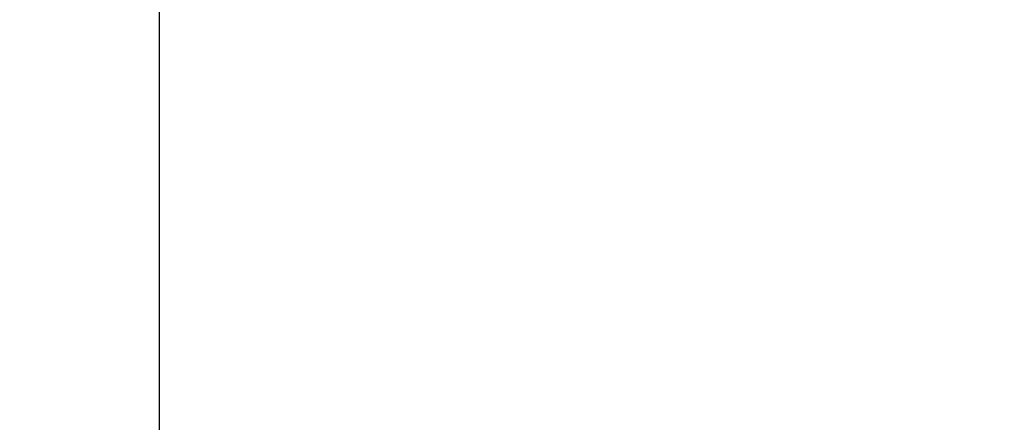
# Model space of a CAD drawing. Units: inches. Extents: x 2091 to 2899, y 967 to 2217.
# Tile 9 of 256: x 2312 to 2351, y 1064 to 1080. Entities that reach past the tile are written whole.
import ezdxf

# ---------------------------------------------------------------- set-up
doc = ezdxf.new("R2010")
doc.units = ezdxf.units.IN
doc.layers.add('A-ANNO-DIMS', color=2, linetype='Continuous', lineweight=18)
doc.styles.get("Standard").update_dxf_attribs({"font": 'arial.ttf'})
doc.dimstyles.new('ISO-25', dxfattribs={"dimtxt": 4, "dimasz": 4, "dimexe": 1.25, "dimexo": 0.625, "dimtad": 1, "dimdec": 0, "dimlunit": 3, "dimtxsty": 'Standard', "dimcen": 2.5, "dimadec": 0, "dimazin": 0, "dimtfac": 1, "dimtdec": 0, "dimtmove": 0, "dimatfit": 3, "dimfxl": 1, "dimarcsym": 0})

# ---------------------------------------------------------------- blocks, each defined once
blk = doc.blocks.new('*D68')
at = {"layer": 'A-ANNO-DIMS', "color": 0, "lineweight": -2, "transparency": 16777216}
for p, q in [((2317.144, 1535.794), (2317.144, 969.464)), ((2459.384, 1535.794), (2459.384, 969.464)), ((2321.144, 970.714), (2455.384, 970.714))]:
    blk.add_line(p, q, dxfattribs=at)
at = {"layer": 'A-ANNO-DIMS', "color": 0, "transparency": 16777216}
for points in [[(2321.144, 971.381), (2321.144, 970.048), (2317.144, 970.714)], [(2455.384, 971.381), (2455.384, 970.048), (2459.384, 970.714)]]:
    blk.add_solid(points, dxfattribs=at)
at = {"layer": 'Defpoints', "color": 0, "transparency": 16777216}
for p in [(2317.144, 1536.419), (2459.384, 1536.419), (2459.384, 970.714)]:
    blk.add_point(p, dxfattribs=at)
at = {"layer": 'A-ANNO-DIMS', "color": 0, "transparency": 16777216, "insert": (2388.264, 973.382), "char_height": 4, "attachment_point": 5}
blk.add_mtext('11\'-10"', dxfattribs=at)
blk = doc.blocks.new('*D71')
at = {"layer": 'A-ANNO-DIMS', "color": 0, "lineweight": -2, "transparency": 16777216}
for p, q in [((2212.144, 1351.294), (2212.144, 969.464)), ((2452.144, 1351.294), (2452.144, 969.464)), ((2216.144, 970.714), (2448.144, 970.714))]:
    blk.add_line(p, q, dxfattribs=at)
at = {"layer": 'A-ANNO-DIMS', "color": 0, "transparency": 16777216}
for points in [[(2216.144, 971.381), (2216.144, 970.048), (2212.144, 970.714)], [(2448.144, 971.381), (2448.144, 970.048), (2452.144, 970.714)]]:
    blk.add_solid(points, dxfattribs=at)
at = {"layer": 'Defpoints', "color": 0, "transparency": 16777216}
for p in [(2212.144, 1351.919), (2452.144, 1351.919), (2452.144, 970.714)]:
    blk.add_point(p, dxfattribs=at)
at = {"layer": 'A-ANNO-DIMS', "color": 0, "transparency": 16777216, "insert": (2332.144, 973.382), "char_height": 4, "attachment_point": 5}
blk.add_mtext('20\'-0"', dxfattribs=at)

msp = doc.modelspace()

# ---------------------------------------------------------------- dimensions: what is measured, and where the dimension line sits
at = {"layer": 'A-ANNO-DIMS'}
for base, p1, p2, picture, middle in [((2459.384, 970.714), (2317.144, 1536.419), (2459.384, 1536.419), '*D68', (2388.264, 973.382)), ((2452.144, 970.714), (2212.144, 1351.919), (2452.144, 1351.919), '*D71', (2332.144, 973.382))]:
    dim = msp.add_linear_dim(base=base, p1=p1, p2=p2, dimstyle='ISO-25', override={"dimdec": 1, "dimlfac": 1, "dimrnd": 0, "dimzin": 1, "dimdsep": 46, "dimlunit": 4, "dimfrac": 2}, dxfattribs=at)
    dim.commit()
    dim.dimension.update_dxf_attribs({"geometry": picture, "text_midpoint": middle})

doc.saveas('drawing.dxf')
